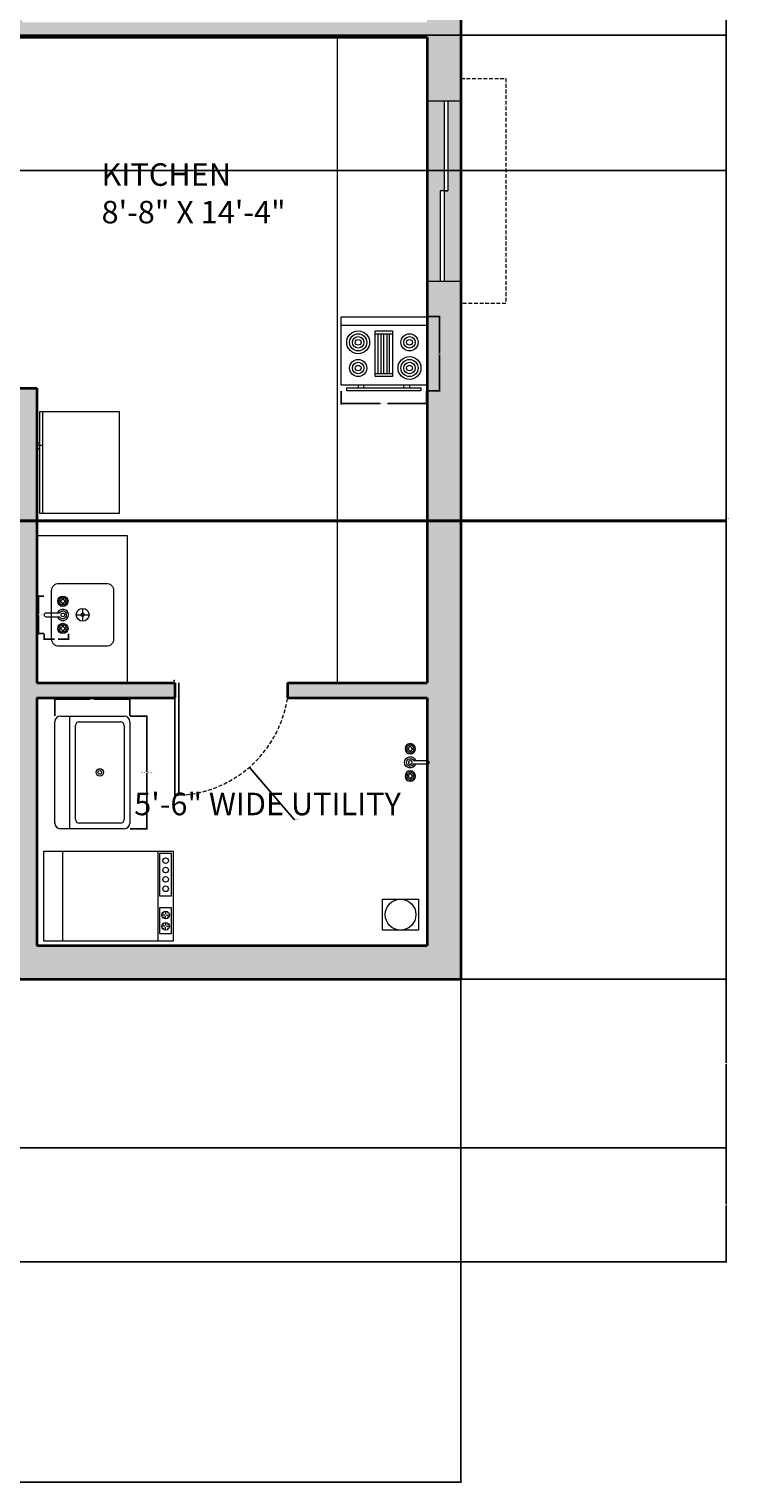
# Model space of a CAD drawing. Units: inches. Extents: x 1693 to 2974, y 2201 to 2965.
# Tile 19 of 24: x 2787 to 2974, y 2201 to 2588. Entities that reach past the tile are written whole.
import ezdxf

# ---------------------------------------------------------------- set-up
doc = ezdxf.new("R2010")
doc.units = ezdxf.units.IN
doc.header["$LTSCALE"] = 2
doc.header["$MEASUREMENT"] = 0
doc.linetypes.add('HIDDEN', pattern=[0.375, 0.25, -0.125])
for name, color, linetype, lineweight in [('A-ANNO-DIMS', 2, 'Continuous', 18), ('A-AREA-IDEN', 7, 'Continuous', 18), ('A-DOOR', 3, 'Continuous', 25), ('A-DOOR-SWNG', 3, 'HIDDEN', 13), ('A-EQPM', 8, 'Continuous', 18), ('A-FLOR-CASE', 32, 'Continuous', 18), ('A-FLOR-FIXT', 9, 'Continuous', 18), ('A-GLAZ', 4, 'Continuous', 18), ('A-GLAZ-OVHD', 8, 'HIDDEN', 13), ('A-WALL', 7, 'Continuous', 35)]:
    doc.layers.add(name, color=color, linetype=linetype, lineweight=lineweight)
doc.layers.add('A-GLAZ-PATT', color=141, linetype='Continuous', lineweight=13, true_color=0xadddf7)
doc.layers.add('A-WALL-PATT', color=251, linetype='Continuous', lineweight=13, true_color=0x636466)
doc.styles.get("Standard").update_dxf_attribs({"font": 'arial.ttf'})
doc.dimstyles.get("Standard").update_dxf_attribs({"dimtxt": 0.18, "dimasz": 0.18, "dimexe": 0.18, "dimexo": 0.0625, "dimgap": 0.09, "dimtad": 0, "dimtih": 1, "dimtoh": 1, "dimdec": 1, "dimzin": 0, "dimdsep": 46, "dimlunit": 3, "dimtxsty": 'Standard', "dimcen": 0.09, "dimadec": 0, "dimazin": 0, "dimtfac": 1, "dimtdec": 1, "dimtofl": 0, "dimtmove": 0, "dimatfit": 3, "dimfxl": 1, "dimtolj": 1, "dimtzin": 0, "dimarcsym": 0})

# ---------------------------------------------------------------- blocks, each defined once
blk = doc.blocks.new('Range-Oven - 30 in top')
for p, q in [((0, -3), (30, -3)), ((12, -6), (18, -6)), ((13, -20), (13, -6)), ((14, -6), (14, -20)), ((15, -20), (15, -6)), ((16, -6), (16, -20)), ((17, -20), (17, -6)), ((18, -20), (12, -20)), ((6, -24), (6, -25)), ((8, -25), (8, -24)), ((22, -25), (22, -24)), ((24, -24), (24, -25))]:
    blk.add_line(p, q)
for points in [[(0, -24), (0, 0), (30, 0), (30, -24)], [(12, -21), (12, -5), (18, -5), (18, -21)], [(2, -26), (2, -25), (28, -25), (28, -26)]]:
    blk.add_lwpolyline(points, close=True)
for centre, radius in [((6, -9), 4), ((6, -9), 3), ((6, -9), 2), ((6, -9), 1), ((24, -9), 3), ((24, -9), 2), ((24, -9), 1), ((6, -18), 3), ((24, -18), 4), ((24, -18), 3), ((6, -18), 2), ((6, -18), 1), ((24, -18), 2), ((24, -18), 1)]:
    blk.add_circle(centre, radius)
blk = doc.blocks.new('Dishwasher')
for p, q in [((16, 32.5), (16.75, 32.5)), ((16.5, 32), (16.2942, 31.7942)), ((16.3156, 33.1843), (16.5, 33)), ((17, 32.75), (17, 33.5)), ((17, 32.25), (17, 31.5)), ((18, 32.5), (17.25, 32.5)), ((17.5, 33), (17.6938, 33.1938)), ((17.7061, 31.7939), (17.5, 32)), ((19, 32.5), (19.75, 32.5)), ((19.5, 32), (19.2942, 31.7942)), ((19.3156, 33.1843), (19.5, 33)), ((20, 32.75), (20, 33.5)), ((20, 32.25), (20, 31.5)), ((21, 32.5), (20.25, 32.5)), ((20.5, 33), (20.6938, 33.1938)), ((20.7061, 31.7939), (20.5, 32)), ((24, 30.5), (0, 30.5)), ((0, 5), (24, 5))]:
    blk.add_line(p, q)
for points in [[(0, 0), (0, 34.5), (24, 34.5), (24, 0)], [(0.5, 31), (0.5, 34), (12, 34), (12, 31)], [(15, 31), (15, 34), (22, 34), (22, 31)]]:
    blk.add_lwpolyline(points, close=True)
for centre, radius in [((2.5, 32.5), 0.75), ((5, 32.5), 0.75), ((7.5, 32.5), 0.75), ((10, 32.5), 0.75), ((17, 32.5), 1), ((20, 32.5), 1)]:
    blk.add_circle(centre, radius)
blk = doc.blocks.new('Sink-single - 30 in top')
blk.add_line((-15, -3.999996), (15, -3.999996))
for points in [[(-13.5, 0), (13.5, 0)], [(-15, -18.499996), (-15, -1.5)], [(15, -1.5), (15, -18.499996)], [(-13.5, -17.499996), (-13.5, -6.499996)], [(-12.5, -5.499996), (12.5, -5.499996)], [(13.5, -6.499996), (13.5, -17.499996)], [(12.5, -18.499996), (-12.5, -18.499996)], [(13.5, -19.999996), (-13.5, -19.999996)]]:
    blk.add_lwpolyline(points)
for radius in [1, 0.5]:
    blk.add_circle((0, -11.999996), radius)
for centre, radius, start, end in [((-13.5, -1.5), 1.5, 90, 180), ((13.5, -1.5), 1.5, 0, 90), ((-12.5, -6.499996), 1, 90, 180), ((12.5, -6.499996), 1, 0, 90), ((-13.5, -18.499996), 1.5, 180, 270), ((-12.5, -17.499996), 1, 180, 270), ((12.5, -17.499996), 1, 270, 0), ((13.5, -18.499996), 1.5, 270, 0)]:
    blk.add_arc(centre, radius, start, end)
blk = doc.blocks.new('Faucet - Bathroom top')
for p, q in [((-4.107, 0.125), (-4.375, 0.125)), ((-3.75, 0.4788), (-3.75, 0.75)), ((-3.5, 0.482), (-3.5, 0.75)), ((-3.1461, 0.125), (-2.875, 0.125)), ((3.143, 0.125), (2.875, 0.125)), ((3.5, 0.4788), (3.5, 0.75)), ((3.75, 0.482), (3.75, 0.75)), ((4.1039, 0.125), (4.375, 0.125)), ((-4.1039, -0.125), (-4.375, -0.125)), ((-3.75, -0.4821), (-3.75, -0.75)), ((-3.5, -0.4789), (-3.5, -0.75)), ((-3.143, -0.125), (-2.875, -0.125)), ((-0.5, -0.8639), (-0.5, -4.5)), ((0.5, -4.5), (0.5, -0.8631)), ((3.1461, -0.125), (2.875, -0.125)), ((3.5, -0.4821), (3.5, -0.75)), ((3.75, -0.4789), (3.75, -0.75)), ((4.107, -0.125), (4.375, -0.125))]:
    blk.add_line(p, q)
for centre, radius in [((-3.625, 0), 1.375), ((-4.625, 0), 0.2795), ((-3.625, 0), 0.5), ((-3.625, 1), 0.2795), ((-2.625, 0), 0.2795), ((0, 0), 0.5), ((3.625, 0), 1.375), ((2.625, 0), 0.2795), ((3.625, 0), 0.5), ((3.625, 1), 0.2795), ((4.625, 0), 0.2795), ((-3.625, -1), 0.2795), ((3.625, -1), 0.2795)]:
    blk.add_circle(centre, radius)
for centre, radius, start, end in [((-3.625, 0), 1, 105.2407, 164.2093), ((-3.625, 0), 1, 16.44125, 74.07887), ((0, 0), 1.5, 289.6514, 250.3603), ((0, 0), 1, 300.3431, 239.7554), ((3.625, 0), 1, 106.12, 164.0884), ((3.625, 0), 1, 16.23422, 73.90469), ((-3.625, 0), 1, 196.2342, 253.9047), ((-3.625, 0), 1, 286.12, 344.0884), ((3.625, 0), 1, 196.4413, 254.0789), ((3.625, 0), 1, 285.2407, 344.2093), ((0, -4.5), 0.5, 180, 0)]:
    blk.add_arc(centre, radius, start, end)
blk = doc.blocks.new('Refrigerator-2 door - 36 in top')
for p, q in [((0, -26.999999), (36, -26.999999)), ((11, -27.999999), (11, -28.999999)), ((11, -28.999999), (13, -28.999999)), ((12, -26.999999), (12, -28.999999)), ((13, -28.999999), (13, -27.999999))]:
    blk.add_line(p, q)
blk.add_lwpolyline([(0, -27.999999), (0, 0), (36, 0), (36, -27.999999)], close=True)
blk = doc.blocks.new('DRAIN-UTILITY')
at = {"ltscale": 2}
blk.add_lwpolyline([(0, 8.21), (9.59, 8.21), (9.59, 0), (0, 0)], close=True, dxfattribs=at)
blk.add_circle((4.8, 4.1), 4.1, dxfattribs=at)
blk = doc.blocks.new('WINDOW-HOOD-60IN')
at = {"ltscale": 2}
for p, q in [((6, 12), (0, 12)), ((0, 12), (0, 0)), ((60, 12), (6, 12)), ((60, 0), (60, 12)), ((54, 0), (60, 0))]:
    blk.add_line(p, q, dxfattribs=at)
blk = doc.blocks.new('*D35')
at = {"layer": 'A-ANNO-DIMS', "color": 0, "lineweight": -2, "ltscale": 2, "transparency": 16777216}
for p, q in [((2791.07, 2436.84), (2789.46, 2436.84)), ((2789.64, 2436.66), (2789.64, 2432.02)), ((2789.64, 2427.02), (2789.64, 2431.66)), ((2791.07, 2426.84), (2789.46, 2426.84))]:
    blk.add_line(p, q, dxfattribs=at)
at = {"layer": 'A-ANNO-DIMS', "color": 0, "ltscale": 2, "transparency": 16777216}
for points in [[(2789.61, 2436.66), (2789.67, 2436.66), (2789.64, 2436.84)], [(2789.61, 2427.02), (2789.67, 2427.02), (2789.64, 2426.84)]]:
    blk.add_solid(points, dxfattribs=at)
at = {"layer": 'Defpoints', "color": 0, "ltscale": 2, "transparency": 16777216}
for p in [(2791.14, 2436.84), (2789.64, 2426.84), (2791.14, 2426.84)]:
    blk.add_point(p, dxfattribs=at)
at = {"layer": 'A-ANNO-DIMS', "color": 0, "ltscale": 2, "transparency": 16777216, "insert": (2789.64, 2431.84), "char_height": 0.18, "attachment_point": 5}
blk.add_mtext('\\A1;TAP - PLAN 10 TYP.', dxfattribs=at)
blk = doc.blocks.new('*D36')
at = {"layer": 'A-ANNO-DIMS', "color": 0, "lineweight": -2, "ltscale": 2, "transparency": 16777216}
for p, q in [((2791.14, 2426.78), (2791.14, 2425.16)), ((2791.32, 2425.34), (2793.93, 2425.34)), ((2797.46, 2425.34), (2794.84, 2425.34)), ((2797.64, 2426.78), (2797.64, 2425.16))]:
    blk.add_line(p, q, dxfattribs=at)
at = {"layer": 'A-ANNO-DIMS', "color": 0, "ltscale": 2, "transparency": 16777216}
for points in [[(2791.32, 2425.37), (2791.32, 2425.31), (2791.14, 2425.34)], [(2797.46, 2425.37), (2797.46, 2425.31), (2797.64, 2425.34)]]:
    blk.add_solid(points, dxfattribs=at)
at = {"layer": 'Defpoints', "color": 0, "ltscale": 2, "transparency": 16777216}
for p in [(2791.14, 2426.84), (2797.64, 2426.84), (2797.64, 2425.34)]:
    blk.add_point(p, dxfattribs=at)
at = {"layer": 'A-ANNO-DIMS', "color": 0, "ltscale": 2, "transparency": 16777216, "insert": (2794.39, 2425.34), "char_height": 0.18, "attachment_point": 5}
blk.add_mtext('\\A1;7 TYP.', dxfattribs=at)
blk = doc.blocks.new('*D53')
at = {"layer": 'A-ANNO-DIMS', "color": 0, "lineweight": -2, "ltscale": 2, "transparency": 16777216}
for p, q in [((2870.29, 2491.47), (2870.29, 2487.94)), ((2893.09, 2491.47), (2893.09, 2487.94)), ((2870.47, 2488.12), (2880.68, 2488.12)), ((2892.91, 2488.12), (2882.69, 2488.12))]:
    blk.add_line(p, q, dxfattribs=at)
at = {"layer": 'A-ANNO-DIMS', "color": 0, "ltscale": 2, "transparency": 16777216}
for points in [[(2870.47, 2488.15), (2870.47, 2488.09), (2870.29, 2488.12)], [(2892.91, 2488.15), (2892.91, 2488.09), (2893.09, 2488.12)]]:
    blk.add_solid(points, dxfattribs=at)
at = {"layer": 'Defpoints', "color": 0, "ltscale": 2, "transparency": 16777216}
for p in [(2870.29, 2491.54), (2893.09, 2491.54), (2893.09, 2488.12)]:
    blk.add_point(p, dxfattribs=at)
at = {"layer": 'A-ANNO-DIMS', "color": 0, "ltscale": 2, "transparency": 16777216, "insert": (2881.69, 2488.12), "char_height": 0.18, "attachment_point": 5}
blk.add_mtext('\\A1;RANGE 23 TYP.', dxfattribs=at)
blk = doc.blocks.new('*D54')
at = {"layer": 'A-ANNO-DIMS', "color": 0, "lineweight": -2, "ltscale": 2, "transparency": 16777216}
for p, q in [((2893.15, 2511.3), (2896.69, 2511.3)), ((2896.51, 2511.12), (2896.51, 2501.6)), ((2896.51, 2491.72), (2896.51, 2501.24)), ((2893.15, 2491.54), (2896.69, 2491.54))]:
    blk.add_line(p, q, dxfattribs=at)
at = {"layer": 'A-ANNO-DIMS', "color": 0, "ltscale": 2, "transparency": 16777216}
for points in [[(2896.48, 2511.12), (2896.54, 2511.12), (2896.51, 2511.3)], [(2896.48, 2491.72), (2896.54, 2491.72), (2896.51, 2491.54)]]:
    blk.add_solid(points, dxfattribs=at)
at = {"layer": 'Defpoints', "color": 0, "ltscale": 2, "transparency": 16777216}
for p in [(2893.09, 2511.3), (2896.51, 2511.3), (2893.09, 2491.54)]:
    blk.add_point(p, dxfattribs=at)
at = {"layer": 'A-ANNO-DIMS', "color": 0, "ltscale": 2, "transparency": 16777216, "insert": (2896.51, 2501.42), "char_height": 0.18, "attachment_point": 5}
blk.add_mtext('\\A1;20 TYP.', dxfattribs=at)
blk = doc.blocks.new('*D59')
at = {"layer": 'A-ANNO-DIMS', "color": 0, "lineweight": -2, "ltscale": 2, "transparency": 16777216}
for p, q in [((2814.04, 2404.86), (2818.66, 2404.86)), ((2818.48, 2404.68), (2818.48, 2390.05)), ((2818.48, 2375.04), (2818.48, 2389.68)), ((2814.04, 2374.86), (2818.66, 2374.86))]:
    blk.add_line(p, q, dxfattribs=at)
at = {"layer": 'A-ANNO-DIMS', "color": 0, "ltscale": 2, "transparency": 16777216}
for points in [[(2818.45, 2404.68), (2818.51, 2404.68), (2818.48, 2404.86)], [(2818.45, 2375.04), (2818.51, 2375.04), (2818.48, 2374.86)]]:
    blk.add_solid(points, dxfattribs=at)
at = {"layer": 'Defpoints', "color": 0, "ltscale": 2, "transparency": 16777216}
for p in [(2813.98, 2404.86), (2818.48, 2404.86), (2813.98, 2374.86)]:
    blk.add_point(p, dxfattribs=at)
at = {"layer": 'A-ANNO-DIMS', "color": 0, "ltscale": 2, "transparency": 16777216, "insert": (2818.48, 2389.86), "char_height": 0.18, "attachment_point": 5}
blk.add_mtext('\\A1;SINGLE-BOWL SINK 30 TYP.', dxfattribs=at)
blk = doc.blocks.new('*D60')
at = {"layer": 'A-ANNO-DIMS', "color": 0, "lineweight": -2, "ltscale": 2, "transparency": 16777216}
for p, q in [((2793.98, 2404.93), (2793.98, 2409.54)), ((2813.98, 2404.93), (2813.98, 2409.54)), ((2794.16, 2409.36), (2803.45, 2409.36)), ((2813.8, 2409.36), (2804.51, 2409.36))]:
    blk.add_line(p, q, dxfattribs=at)
at = {"layer": 'A-ANNO-DIMS', "color": 0, "ltscale": 2, "transparency": 16777216}
for points in [[(2794.16, 2409.39), (2794.16, 2409.33), (2793.98, 2409.36)], [(2813.8, 2409.39), (2813.8, 2409.33), (2813.98, 2409.36)]]:
    blk.add_solid(points, dxfattribs=at)
at = {"layer": 'Defpoints', "color": 0, "ltscale": 2, "transparency": 16777216}
for p in [(2793.98, 2409.36), (2793.98, 2404.86), (2813.98, 2404.86)]:
    blk.add_point(p, dxfattribs=at)
at = {"layer": 'A-ANNO-DIMS', "color": 0, "ltscale": 2, "transparency": 16777216, "insert": (2803.98, 2409.36), "char_height": 0.18, "attachment_point": 5}
blk.add_mtext('\\A1;20 TYP.', dxfattribs=at)
blk = doc.blocks.new('*D81')
at = {"layer": 'A-ANNO-DIMS', "color": 0, "lineweight": -2, "ltscale": 2, "transparency": 16777216}
for p, q in [((1752.34, 2553.91), (1752.34, 2964.96)), ((1752.52, 2964.78), (2332.94, 2964.78)), ((2914.06, 2964.78), (2333.64, 2964.78)), ((2914.24, 2754.97), (2914.24, 2964.96))]:
    blk.add_line(p, q, dxfattribs=at)
at = {"layer": 'A-ANNO-DIMS', "color": 0, "ltscale": 2, "transparency": 16777216}
for points in [[(1752.52, 2964.81), (1752.52, 2964.75), (1752.34, 2964.78)], [(2914.06, 2964.81), (2914.06, 2964.75), (2914.24, 2964.78)]]:
    blk.add_solid(points, dxfattribs=at)
at = {"layer": 'Defpoints', "color": 0, "ltscale": 2, "transparency": 16777216}
for p in [(2914.24, 2964.78), (2914.24, 2754.9), (1752.34, 2553.84)]:
    blk.add_point(p, dxfattribs=at)
at = {"layer": 'A-ANNO-DIMS', "color": 0, "ltscale": 2, "transparency": 16777216, "insert": (2333.29, 2964.78), "char_height": 0.18, "attachment_point": 5}
blk.add_mtext('\\A1;1162', dxfattribs=at)
blk = doc.blocks.new('*D85')
at = {"layer": 'A-ANNO-DIMS', "color": 0, "lineweight": -2, "ltscale": 2, "transparency": 16777216}
for p, q in [((2479.24, 2334.69), (2479.24, 2200.56)), ((2902.24, 2334.69), (2902.24, 2200.56)), ((2479.42, 2200.74), (2690.44, 2200.74)), ((2902.06, 2200.74), (2691.03, 2200.74))]:
    blk.add_line(p, q, dxfattribs=at)
at = {"layer": 'A-ANNO-DIMS', "color": 0, "ltscale": 2, "transparency": 16777216}
for points in [[(2479.42, 2200.77), (2479.42, 2200.71), (2479.24, 2200.74)], [(2902.06, 2200.77), (2902.06, 2200.71), (2902.24, 2200.74)]]:
    blk.add_solid(points, dxfattribs=at)
at = {"layer": 'Defpoints', "color": 0, "ltscale": 2, "transparency": 16777216}
for p in [(2479.24, 2334.75), (2902.24, 2334.75), (2902.24, 2200.74)]:
    blk.add_point(p, dxfattribs=at)
at = {"layer": 'A-ANNO-DIMS', "color": 0, "ltscale": 2, "transparency": 16777216, "insert": (2690.74, 2200.74), "char_height": 0.18, "attachment_point": 5}
blk.add_mtext('\\A1;423', dxfattribs=at)
blk = doc.blocks.new('*D87')
at = {"layer": 'A-ANNO-DIMS', "color": 0, "lineweight": -2, "ltscale": 2, "transparency": 16777216}
for p, q in [((2902.3, 2846.25), (2973.12, 2846.25)), ((2972.94, 2846.07), (2972.94, 2590.69)), ((2972.94, 2334.93), (2972.94, 2590.32)), ((2902.3, 2334.75), (2973.12, 2334.75))]:
    blk.add_line(p, q, dxfattribs=at)
at = {"layer": 'A-ANNO-DIMS', "color": 0, "ltscale": 2, "transparency": 16777216}
for points in [[(2972.91, 2846.07), (2972.97, 2846.07), (2972.94, 2846.25)], [(2972.91, 2334.93), (2972.97, 2334.93), (2972.94, 2334.75)]]:
    blk.add_solid(points, dxfattribs=at)
at = {"layer": 'Defpoints', "color": 0, "ltscale": 2, "transparency": 16777216}
for p in [(2902.24, 2846.25), (2972.94, 2846.25), (2902.24, 2334.75)]:
    blk.add_point(p, dxfattribs=at)
at = {"layer": 'A-ANNO-DIMS', "color": 0, "ltscale": 2, "transparency": 16777216, "insert": (2972.94, 2590.5), "char_height": 0.18, "attachment_point": 5}
blk.add_mtext('\\A1;511.5', dxfattribs=at)
blk = doc.blocks.new('*D89')
at = {"layer": 'A-ANNO-DIMS', "color": 0, "lineweight": -2, "ltscale": 2, "transparency": 16777216}
for p, q in [((2479.3, 2334.75), (2973.12, 2334.75)), ((2972.94, 2334.57), (2972.94, 2312.48)), ((2972.94, 2290.02), (2972.94, 2312.12)), ((2294.3, 2289.84), (2973.12, 2289.84))]:
    blk.add_line(p, q, dxfattribs=at)
at = {"layer": 'A-ANNO-DIMS', "color": 0, "ltscale": 2, "transparency": 16777216}
for points in [[(2972.91, 2334.57), (2972.97, 2334.57), (2972.94, 2334.75)], [(2972.91, 2290.02), (2972.97, 2290.02), (2972.94, 2289.84)]]:
    blk.add_solid(points, dxfattribs=at)
at = {"layer": 'Defpoints', "color": 0, "ltscale": 2, "transparency": 16777216}
for p in [(2479.24, 2334.75), (2972.94, 2334.75), (2294.24, 2289.84)]:
    blk.add_point(p, dxfattribs=at)
at = {"layer": 'A-ANNO-DIMS', "color": 0, "ltscale": 2, "transparency": 16777216, "insert": (2972.94, 2312.3), "char_height": 0.18, "attachment_point": 5}
blk.add_mtext('\\A1;44.91', dxfattribs=at)
blk = doc.blocks.new('*D95')
at = {"layer": 'A-ANNO-DIMS', "color": 0, "lineweight": -2, "ltscale": 2, "transparency": 16777216}
for p, q in [((2189.3, 2289.84), (2973.12, 2289.84)), ((2972.94, 2289.66), (2972.94, 2274.83)), ((2972.94, 2259.62), (2972.94, 2274.46)), ((2189.3, 2259.44), (2973.12, 2259.44))]:
    blk.add_line(p, q, dxfattribs=at)
at = {"layer": 'A-ANNO-DIMS', "color": 0, "ltscale": 2, "transparency": 16777216}
for points in [[(2972.91, 2289.66), (2972.97, 2289.66), (2972.94, 2289.84)], [(2972.91, 2259.62), (2972.97, 2259.62), (2972.94, 2259.44)]]:
    blk.add_solid(points, dxfattribs=at)
at = {"layer": 'Defpoints', "color": 0, "ltscale": 2, "transparency": 16777216}
for p in [(2189.24, 2289.84), (2972.94, 2289.84), (2189.24, 2259.44)]:
    blk.add_point(p, dxfattribs=at)
at = {"layer": 'A-ANNO-DIMS', "color": 0, "ltscale": 2, "transparency": 16777216, "insert": (2972.94, 2274.64), "char_height": 0.18, "attachment_point": 5}
blk.add_mtext('\\A1;30.4', dxfattribs=at)
blk = doc.blocks.new('*D96')
at = {"layer": 'A-ANNO-DIMS', "color": 0, "lineweight": -2, "ltscale": 2, "transparency": 16777216}
for p, q in [((2294.3, 2586.26), (2973.12, 2586.26)), ((2972.94, 2586.08), (2972.94, 2568.45)), ((2972.94, 2550.44), (2972.94, 2568.08)), ((2294.3, 2550.26), (2973.12, 2550.26))]:
    blk.add_line(p, q, dxfattribs=at)
at = {"layer": 'A-ANNO-DIMS', "color": 0, "ltscale": 2, "transparency": 16777216}
for points in [[(2972.91, 2586.08), (2972.97, 2586.08), (2972.94, 2586.26)], [(2972.91, 2550.44), (2972.97, 2550.44), (2972.94, 2550.26)]]:
    blk.add_solid(points, dxfattribs=at)
at = {"layer": 'Defpoints', "color": 0, "ltscale": 2, "transparency": 16777216}
for p in [(2294.24, 2586.26), (2972.94, 2586.26), (2294.24, 2550.26)]:
    blk.add_point(p, dxfattribs=at)
at = {"layer": 'A-ANNO-DIMS', "color": 0, "ltscale": 2, "transparency": 16777216, "insert": (2972.94, 2568.26), "char_height": 0.18, "attachment_point": 5}
blk.add_mtext('\\A1;36', dxfattribs=at)
blk = doc.blocks.new('*D97')
at = {"layer": 'A-ANNO-DIMS', "color": 0, "lineweight": -2, "ltscale": 2, "transparency": 16777216}
for p, q in [((2294.3, 2631.75), (2973.12, 2631.75)), ((2972.94, 2631.57), (2972.94, 2609.19)), ((2972.94, 2586.44), (2972.94, 2608.83)), ((2294.3, 2586.26), (2973.12, 2586.26))]:
    blk.add_line(p, q, dxfattribs=at)
at = {"layer": 'A-ANNO-DIMS', "color": 0, "ltscale": 2, "transparency": 16777216}
for points in [[(2972.91, 2631.57), (2972.97, 2631.57), (2972.94, 2631.75)], [(2972.91, 2586.44), (2972.97, 2586.44), (2972.94, 2586.26)]]:
    blk.add_solid(points, dxfattribs=at)
at = {"layer": 'Defpoints', "color": 0, "ltscale": 2, "transparency": 16777216}
for p in [(2294.24, 2631.75), (2972.94, 2631.75), (2294.24, 2586.26)]:
    blk.add_point(p, dxfattribs=at)
at = {"layer": 'A-ANNO-DIMS', "color": 0, "ltscale": 2, "transparency": 16777216, "insert": (2972.94, 2609.01), "char_height": 0.18, "attachment_point": 5}
blk.add_mtext('\\A1;45.49', dxfattribs=at)
blk = doc.blocks.new('*D108')
at = {"layer": 'A-ANNO-DIMS', "color": 0, "lineweight": -2, "ltscale": 2, "transparency": 16777216}
for p, q in [((1752.74, 2457.09), (2973.12, 2457.09)), ((1752.74, 2456.73), (2973.12, 2456.73)), ((2972.94, 2457.27), (2972.94, 2457.45)), ((2972.94, 2457.45), (2973.12, 2457.45)), ((2972.94, 2456.55), (2972.94, 2456.37))]:
    blk.add_line(p, q, dxfattribs=at)
at = {"layer": 'A-ANNO-DIMS', "color": 0, "ltscale": 2, "transparency": 16777216}
for points in [[(2972.91, 2457.27), (2972.97, 2457.27), (2972.94, 2457.09)], [(2972.91, 2456.55), (2972.97, 2456.55), (2972.94, 2456.73)]]:
    blk.add_solid(points, dxfattribs=at)
at = {"layer": 'Defpoints', "color": 0, "ltscale": 2, "transparency": 16777216}
for p in [(1752.68, 2457.09), (1752.68, 2456.73), (2972.94, 2457.09)]:
    blk.add_point(p, dxfattribs=at)
at = {"layer": 'A-ANNO-DIMS', "color": 0, "ltscale": 2, "transparency": 16777216, "insert": (2973.44, 2457.45), "char_height": 0.18, "attachment_point": 5}
blk.add_mtext('\\A1;0.36', dxfattribs=at)
blk = doc.blocks.new('*D119')
at = {"layer": 'A-ANNO-DIMS', "color": 0, "lineweight": -2, "ltscale": 2, "transparency": 16777216}
for p, q in [((2825.7, 2414.32), (2825.88, 2414.32)), ((2825.79, 2414.23), (2825.79, 2414.41)), ((2857.82, 2377.36), (2845.93, 2391.09)), ((2858, 2377.36), (2857.82, 2377.36))]:
    blk.add_line(p, q, dxfattribs=at)
at = {"layer": 'A-ANNO-DIMS', "color": 0, "ltscale": 2, "transparency": 16777216}
blk.add_solid([(2845.95, 2391.11), (2845.91, 2391.07), (2845.81, 2391.22)], dxfattribs=at)
at = {"layer": 'Defpoints', "color": 0, "ltscale": 2, "transparency": 16777216}
for p in [(2825.79, 2414.32), (2845.81, 2391.22)]:
    blk.add_point(p, dxfattribs=at)
at = {"layer": 'A-ANNO-DIMS', "color": 0, "ltscale": 2, "transparency": 16777216, "insert": (2858.55, 2377.36), "char_height": 0.18, "attachment_point": 5}
blk.add_mtext('\\A1;R30.567', dxfattribs=at)

msp = doc.modelspace()

# ---------------------------------------------------------------- hatches: boundary and pattern name
at = {"layer": 'A-GLAZ-PATT', "ltscale": 2}
h = msp.add_hatch(color=256, dxfattribs=at)
h.dxf.hatch_style = 1
h.paths.add_polyline_path([(2656.9702, 2338.2547), (2632.9702, 2338.2547), (2632.9702, 2339.2547), (2608.9702, 2339.2547), (2608.9702, 2334.7547), (2656.9702, 2334.7547)])
h.paths.add_polyline_path([(2656.9702, 2343.7547), (2608.9702, 2343.7547), (2608.9702, 2340.2547), (2632.9702, 2340.2547), (2632.9702, 2339.2547), (2656.9702, 2339.2547)])
h.paths.add_polyline_path([(2775.7544, 2338.2547), (2751.7544, 2338.2547), (2751.7544, 2334.7547), (2775.7544, 2334.7547)])
h.paths.add_polyline_path([(2775.7544, 2343.7547), (2751.7544, 2343.7547), (2751.7544, 2340.2547), (2775.7544, 2340.2547)])
h.paths.add_polyline_path([(2897.7363, 2568.7999), (2893.2363, 2568.7999), (2893.2363, 2520.7999), (2896.7363, 2520.7999), (2896.7363, 2544.7999), (2897.7363, 2544.7999)])
h.paths.add_polyline_path([(2902.2363, 2568.7999), (2898.7363, 2568.7999), (2898.7363, 2544.7999), (2897.7363, 2544.7999), (2897.7363, 2520.7999), (2902.2363, 2520.7999)])
h.paths.add_polyline_path([(2902.2363, 2637.7547), (2898.7363, 2637.7547), (2898.7363, 2613.7547), (2902.2363, 2613.7547)])
h.paths.add_polyline_path([(2896.7363, 2637.7547), (2893.2363, 2637.7547), (2893.2363, 2613.7547), (2896.7363, 2613.7547)])
h.paths.add_polyline_path([(2902.2363, 2748.903), (2899.0477, 2748.903), (2899.0477, 2724.903), (2898.0477, 2724.903), (2898.0477, 2700.903), (2902.2363, 2700.903)])
h.paths.add_polyline_path([(2898.0477, 2748.903), (2893.2363, 2748.903), (2893.2363, 2700.903), (2897.0477, 2700.903), (2897.0477, 2724.903), (2898.0477, 2724.903)])
h.paths.add_polyline_path([(2851.2363, 2846.2547), (2803.2363, 2846.2547), (2803.2363, 2842.7547), (2827.2363, 2842.7547), (2827.2363, 2841.7547), (2851.2363, 2841.7547)])
h.paths.add_polyline_path([(2851.2363, 2840.7547), (2827.2363, 2840.7547), (2827.2363, 2841.7547), (2803.2363, 2841.7547), (2803.2363, 2837.2547), (2851.2363, 2837.2547)])
h.paths.add_polyline_path([(2578.2363, 2846.2547), (2530.2363, 2846.2547), (2530.2363, 2842.7547), (2554.2363, 2842.7547), (2554.2363, 2841.7547), (2578.2363, 2841.7547)])
h.paths.add_polyline_path([(2578.2363, 2840.7547), (2554.2363, 2840.7547), (2554.2363, 2841.7547), (2530.2363, 2841.7547), (2530.2363, 2837.2547), (2578.2363, 2837.2547)])
h.paths.add_polyline_path([(2732.7363, 2812.7547), (2705.1363, 2812.7547), (2705.1363, 2811.7547), (2676.3363, 2811.7547), (2676.3363, 2812.7547), (2648.7363, 2812.7547), (2648.7363, 2808.2547), (2732.7363, 2808.2547)])
h.paths.add_polyline_path([(2732.7363, 2817.2547), (2648.7363, 2817.2547), (2648.7363, 2813.7547), (2676.3363, 2813.7547), (2676.3363, 2812.7547), (2705.1363, 2812.7547), (2705.1363, 2813.7547), (2732.7363, 2813.7547)])
h.paths.add_polyline_path([(2488.2363, 2695.8203), (2484.7878, 2695.8203), (2484.7878, 2671.8203), (2488.2363, 2671.8203)])
h.paths.add_polyline_path([(2482.7878, 2695.8203), (2479.2363, 2695.8203), (2479.2363, 2671.8203), (2482.7878, 2671.8203)])
h.paths.add_polyline_path([(2488.2363, 2572.4371), (2484.7363, 2572.4371), (2484.7363, 2541.4371), (2483.7363, 2541.4371), (2483.7363, 2512.4371), (2488.2363, 2512.4371)])
h.paths.add_polyline_path([(2482.7363, 2541.4371), (2483.7363, 2541.4371), (2483.7363, 2572.4371), (2479.2363, 2572.4371), (2479.2363, 2512.4371), (2482.7363, 2512.4371)])
h.paths.add_polyline_path([(2248.9863, 2706.8449), (2190.9863, 2706.8449), (2190.9863, 2703.3449), (2219.9863, 2703.3449), (2219.9863, 2702.3449), (2248.9863, 2702.3449)])
h.paths.add_polyline_path([(2248.9863, 2701.3449), (2219.9863, 2701.3449), (2219.9863, 2702.3449), (2190.9863, 2702.3449), (2190.9863, 2697.8449), (2248.9863, 2697.8449)])
h.paths.add_polyline_path([(2151.9207, 2293.3449), (2127.9207, 2293.3449), (2127.9207, 2289.8449), (2151.9207, 2289.8449)])
h.paths.add_polyline_path([(2151.9207, 2298.8449), (2127.9207, 2298.8449), (2127.9207, 2295.3449), (2151.9207, 2295.3449)])
h.paths.add_polyline_path([(2084.023, 2293.3449), (2066.023, 2293.3449), (2066.023, 2294.3449), (2048.023, 2294.3449), (2048.023, 2289.8449), (2084.023, 2289.8449)])
h.paths.add_polyline_path([(2084.023, 2298.8449), (2048.023, 2298.8449), (2048.023, 2295.3449), (2066.023, 2295.3449), (2066.023, 2294.3449), (2084.023, 2294.3449)])
h.paths.add_polyline_path([(1966.0781, 2293.3449), (1948.0781, 2293.3449), (1948.0781, 2294.3449), (1930.0781, 2294.3449), (1930.0781, 2289.8449), (1966.0781, 2289.8449)])
h.paths.add_polyline_path([(1966.0781, 2298.8449), (1930.0781, 2298.8449), (1930.0781, 2295.3449), (1948.0781, 2295.3449), (1948.0781, 2294.3449), (1966.0781, 2294.3449)])
h.paths.add_polyline_path([(1787.2363, 2403.1922), (1782.7363, 2403.1922), (1782.7363, 2355.1922), (1786.2363, 2355.1922), (1786.2363, 2379.1922), (1787.2363, 2379.1922)])
h.paths.add_polyline_path([(1791.7363, 2403.1922), (1788.2363, 2403.1922), (1788.2363, 2379.1922), (1787.2363, 2379.1922), (1787.2363, 2355.1922), (1791.7363, 2355.1922)])
h.paths.add_polyline_path([(1786.2363, 2477.5455), (1782.7363, 2477.5455), (1782.7363, 2453.5455), (1786.2363, 2453.5455)])
h.paths.add_polyline_path([(1791.7363, 2477.5455), (1788.2363, 2477.5455), (1788.2363, 2453.5455), (1791.7363, 2453.5455)])
h.paths.add_polyline_path([(1786.2363, 2621.6433), (1782.7363, 2621.6433), (1782.7363, 2585.6433), (1786.2363, 2585.6433)])
h.paths.add_polyline_path([(1791.7363, 2621.6433), (1788.2363, 2621.6433), (1788.2363, 2585.6433), (1791.7363, 2585.6433)])
h.paths.add_polyline_path([(1908.1286, 2706.8449), (1860.1286, 2706.8449), (1860.1286, 2703.3449), (1884.1286, 2703.3449), (1884.1286, 2702.3449), (1908.1286, 2702.3449)])
h.paths.add_polyline_path([(1908.1286, 2701.3449), (1884.1286, 2701.3449), (1884.1286, 2702.3449), (1860.1286, 2702.3449), (1860.1286, 2697.8449), (1908.1286, 2697.8449)])
h.paths.add_polyline_path([(1973.9863, 2706.8449), (1949.9863, 2706.8449), (1949.9863, 2703.3449), (1973.9863, 2703.3449)])
h.paths.add_polyline_path([(1973.9863, 2701.3449), (1949.9863, 2701.3449), (1949.9863, 2697.8449), (1973.9863, 2697.8449)])
h.paths.add_polyline_path([(2112.7363, 2690.3449), (2028.7363, 2690.3449), (2028.7363, 2686.8449), (2056.3363, 2686.8449), (2056.3363, 2685.8449), (2085.1363, 2685.8449), (2085.1363, 2686.8449), (2112.7363, 2686.8449)])
h.paths.add_polyline_path([(2112.7363, 2685.8449), (2085.1363, 2685.8449), (2085.1363, 2684.8449), (2056.3363, 2684.8449), (2056.3363, 2685.8449), (2028.7363, 2685.8449), (2028.7363, 2681.3449), (2112.7363, 2681.3449)])
h.paths.add_polyline_path([(2422.7363, 2640.7547), (2350.7363, 2640.7547), (2350.7363, 2637.2547), (2386.7363, 2637.2547), (2386.7363, 2636.2547), (2422.7363, 2636.2547)])
h.paths.add_polyline_path([(2422.7363, 2635.2547), (2386.7363, 2635.2547), (2386.7363, 2636.2547), (2350.7363, 2636.2547), (2350.7363, 2631.7547), (2422.7363, 2631.7547)])
at = {"layer": 'A-WALL-PATT', "ltscale": 2}
h = msp.add_hatch(color=256, dxfattribs=at)
h.dxf.hatch_style = 1
h.paths.add_polyline_path([(1928.2363, 2733.2161), (1930.9384, 2733.2161), (1930.9384, 2737.2161), (1923.7363, 2737.2161), (1923.7363, 2706.8449), (1908.1286, 2706.8449), (1908.1286, 2697.8449), (1923.7363, 2697.8449), (1923.7363, 2692.8449), (1928.2363, 2692.8449), (1928.2363, 2697.8449), (1949.9863, 2697.8449), (1949.9863, 2706.8449), (1928.2363, 2706.8449)])
h.paths.add_polyline_path([(2004.7363, 2737.2161), (1995.7363, 2737.2161), (1995.7363, 2706.8449), (1985.6374, 2706.8449), (1973.9863, 2706.8449), (1973.9863, 2697.8449), (2000.2363, 2697.8449), (2000.2363, 2686.5348), (2000.3613, 2686.5348), (2000.3613, 2667.0432), (2000.2363, 2601.8449), (1928.2363, 2601.8449), (1928.2363, 2662.8449), (1923.7363, 2662.8449), (1923.7363, 2595.3449), (1928.2363, 2595.3449), (1928.2363, 2597.3449), (2004.7363, 2597.3449), (2004.7363, 2681.3449), (2012.7814, 2681.3449), (2028.7363, 2681.3449), (2028.7363, 2690.3449), (2004.7363, 2690.3449)])
h.paths.add_polyline_path([(2190.9863, 2706.8449), (2184.9863, 2706.8449), (2145.7363, 2706.8449), (2145.7363, 2765.3449), (2145.7363, 2774.5394), (2136.7363, 2774.5394), (2136.7363, 2756.3449), (2136.7363, 2690.3449), (2112.7363, 2690.3449), (2112.7363, 2681.3449), (2136.7363, 2681.3449), (2136.7363, 2597.3449), (2141.2363, 2597.3449), (2141.2363, 2697.8449), (2190.9863, 2697.8449)])
h.paths.add_polyline_path([(1860.1286, 2706.8449), (1782.7363, 2706.8449), (1782.7363, 2621.6433), (1791.7363, 2621.6433), (1791.7363, 2697.8449), (1860.1286, 2697.8449)])
h.paths.add_polyline_path([(1791.7363, 2585.6433), (1782.7363, 2585.6433), (1782.7363, 2562.8449), (1782.7363, 2553.8449), (1752.3363, 2553.8449), (1752.3363, 2544.2586), (1756.3363, 2544.2586), (1756.3363, 2549.3449), (1782.7363, 2549.3449), (1782.7363, 2489.2404), (1782.7363, 2477.5455), (1791.7363, 2477.5455), (1791.7363, 2493.5991), (1791.6113, 2493.5991), (1791.6113, 2513.0907), (1791.6824, 2533.7198, -0.94742783), (1791.7363, 2534.7168), (1791.7363, 2549.3449), (1863.7363, 2549.3449), (1863.7363, 2513.3449), (1866.7363, 2513.3449), (1866.7363, 2549.3449), (1924.7363, 2549.3449), (1924.7363, 2447.3449), (1924.7363, 2442.8449), (1933.7363, 2442.8449), (1933.7363, 2447.3449), (1928.2363, 2447.3449), (1928.2363, 2559.3449), (1923.7363, 2559.3449), (1923.7363, 2553.8449), (1791.7363, 2553.8449), (1791.7363, 2562.8449)])
h.paths.add_polyline_path([(1791.7363, 2442.8449), (1866.7363, 2442.8449), (1866.7363, 2447.3449), (1866.7363, 2483.3449), (1863.7363, 2483.3449), (1863.7363, 2447.3449), (1791.7363, 2447.3449), (1791.7363, 2453.5455), (1782.7363, 2453.5455), (1782.7363, 2447.3449), (1756.3363, 2447.3449), (1756.3363, 2455.7126), (1752.3363, 2455.7126), (1752.3363, 2442.8449), (1782.7363, 2442.8449), (1782.7363, 2403.1922), (1791.7363, 2403.1922)])
h.paths.add_polyline_path([(1930.0781, 2298.8449), (1791.7363, 2298.8449), (1791.7363, 2355.1922), (1782.7363, 2355.1922), (1782.7363, 2289.8449), (1930.0781, 2289.8449)])
h.paths.add_polyline_path([(2624.7363, 2883.2547), (2624.7363, 2902.6165), (2624.7363, 2906.0761), (2615.7363, 2906.0761), (2615.7363, 2892.2547), (2615.7363, 2846.2547), (2578.2363, 2846.2547), (2578.2363, 2837.2547), (2620.2363, 2837.2547), (2620.2363, 2743.2547), (2624.7363, 2743.2547), (2624.7363, 2808.2547), (2648.7363, 2808.2547), (2648.7363, 2817.2547), (2624.7363, 2817.2547)])
h.paths.add_polyline_path([(2530.2363, 2846.2547), (2479.2363, 2846.2547), (2479.2363, 2695.8203), (2488.2363, 2695.8203), (2488.2363, 2700.7547), (2567.2363, 2700.7547), (2567.2363, 2705.2547), (2488.2363, 2705.2547), (2488.2363, 2837.2547), (2530.2363, 2837.2547)])
h.paths.add_polyline_path([(2488.2363, 2487.7547), (2630.2363, 2487.7547, -0.00990191), (2630.2363, 2489.0322), (2630.2363, 2492.2547), (2488.2363, 2492.2547), (2488.2363, 2512.4371), (2479.2363, 2512.4371), (2479.2363, 2334.7547), (2608.9702, 2334.7547), (2608.9702, 2343.7547), (2488.2363, 2343.7547)])
h.paths.add_polyline_path([(2751.7544, 2343.7547), (2672.7363, 2343.7547), (2672.7363, 2409.7547), (2674.7363, 2409.7547), (2674.7363, 2413.7547), (2672.7363, 2413.7547), (2672.7363, 2487.7547), (2732.7363, 2487.7547), (2732.7363, 2413.7547), (2704.7363, 2413.7547), (2704.7363, 2409.7547), (2784.7363, 2409.7547), (2784.7363, 2343.7547), (2775.7544, 2343.7547), (2775.7544, 2334.7547), (2902.2363, 2334.7547), (2902.2363, 2520.7999), (2893.2363, 2520.7999), (2893.2363, 2413.7547), (2856.0145, 2413.7547), (2856.0145, 2409.7547), (2893.2363, 2409.7547), (2893.2363, 2343.7547), (2789.2363, 2343.7547), (2789.2363, 2409.7547), (2819.2363, 2409.7547), (2826.0145, 2409.7547), (2826.0145, 2413.7547), (2789.2363, 2413.7547), (2789.2363, 2492.2547), (2784.7363, 2492.2547), (2784.7363, 2413.7547), (2736.7363, 2413.7547), (2736.7363, 2492.2547), (2672.7363, 2492.2547), (2666.2363, 2492.2547), (2666.2363, 2487.7547), (2668.2363, 2487.7547), (2668.2363, 2343.7547), (2656.9702, 2343.7547), (2656.9702, 2334.7547), (2662.9702, 2334.7547), (2751.7544, 2334.7547)])
h.paths.add_polyline_path([(2902.2363, 2613.7547), (2893.2363, 2613.7547), (2893.2363, 2589.7547), (2785.2363, 2589.7547), (2785.2363, 2661.7547), (2790.2363, 2661.7547), (2790.2363, 2665.2547), (2761.2363, 2665.2547), (2761.2363, 2667.2547), (2756.7363, 2667.2547), (2756.7363, 2661.7547), (2781.2363, 2661.7547), (2781.2363, 2585.7547), (2893.2363, 2585.7547), (2893.2363, 2568.7999), (2902.2363, 2568.7999)])
h.paths.add_polyline_path([(2488.2363, 2671.8203), (2479.2363, 2671.8203), (2479.2363, 2645.2547), (2479.2363, 2623.4598), (2488.2363, 2623.4598), (2488.2363, 2636.2547), (2624.7363, 2636.2547), (2624.7363, 2640.7547), (2603.7363, 2640.7547), (2603.7363, 2700.7547), (2624.7363, 2700.7547), (2624.7363, 2707.2547), (2620.2363, 2707.2547), (2620.2363, 2705.2547), (2597.2363, 2705.2547), (2597.2363, 2700.7547), (2599.2363, 2700.7547), (2599.2363, 2640.7547), (2488.2363, 2640.7547)])
h.paths.add_polyline_path([(2761.2363, 2837.2547), (2803.2363, 2837.2547), (2803.2363, 2846.2547), (2797.2363, 2846.2547), (2765.7363, 2846.2547), (2756.7363, 2846.2547), (2756.7363, 2817.2547), (2732.7363, 2817.2547), (2732.7363, 2808.2547), (2756.7363, 2808.2547), (2756.7363, 2703.2547), (2761.2363, 2703.2547)])
h.paths.add_polyline_path([(2739.7489, 2433.1234), (2786.9181, 2433.1234), (2786.9181, 2455.5122), (2739.7489, 2455.5122)], flags=25)

# ---------------------------------------------------------------- linework, layer by layer
at = {"layer": 'A-DOOR', "ltscale": 2}
for p, q in [((2826.0145, 2413.7547), (2826.0145, 2383.7547)), ((2827.0145, 2413.7547), (2827.0145, 2383.7547))]:
    msp.add_line(p, q, dxfattribs=at)
at = {"layer": 'A-DOOR-SWNG', "ltscale": 2}
msp.add_arc((2825.7908, 2414.3205), 30.5667, 270.419369, 351.409397, dxfattribs=at)
at = {"layer": 'A-FLOR-CASE'}
for p, q in [((2869.2363, 2585.7547), (2869.2363, 2413.7547)), ((2813.2363, 2453.0047), (2813.2363, 2413.7547))]:
    msp.add_line(p, q, dxfattribs=at)
at = {"layer": 'A-FLOR-CASE', "ltscale": 2}
msp.add_line((2789.2363, 2453.0047), (2813.2363, 2453.0047), dxfattribs=at)
at = {"layer": 'A-FLOR-FIXT', "ltscale": 2}
for p, q in [((2801.4038, 2433.5552), (2801.4038, 2430.1624)), ((2799.7074, 2431.8588), (2803.1002, 2431.8588))]:
    msp.add_line(p, q, dxfattribs=at)
msp.add_lwpolyline([(2795.1387, 2440.2493), (2807.6689, 2440.2493, -0.41421356), (2809.6689, 2438.2493), (2809.6689, 2425.4683, -0.41421356), (2807.6689, 2423.4683), (2795.1387, 2423.4683, -0.41421356), (2793.1387, 2425.4683), (2793.1387, 2438.2493, -0.41421356)], format="xyb", close=True, dxfattribs=at)
for radius in [1.6964, 0.4868]:
    msp.add_circle((2801.4038, 2431.8588), radius, dxfattribs=at)
at = {"layer": 'A-GLAZ', "ltscale": 2}
for p, q in [((2893.2363, 2568.7999), (2902.2363, 2568.7999)), ((2897.7363, 2568.7999), (2897.7363, 2520.7999)), ((2898.7363, 2568.7999), (2898.7363, 2544.7999)), ((2896.7363, 2544.7999), (2896.7363, 2520.7999)), ((2898.7363, 2544.7999), (2896.7363, 2544.7999)), ((2897.7363, 2544.7999), (2898.7363, 2544.7999)), ((2893.2363, 2520.7999), (2902.2363, 2520.7999))]:
    msp.add_line(p, q, dxfattribs=at)
at = {"layer": 'A-WALL'}
for p, q in [((2902.2363, 2846.2547), (2902.2363, 2334.7547)), ((2893.2363, 2585.7547), (2893.2363, 2413.7547)), ((2789.2363, 2492.2547), (2789.2363, 2413.7547)), ((2789.2363, 2409.7547), (2789.2363, 2343.7547)), ((2789.2363, 2409.7547), (2819.2363, 2409.7547)), ((2893.2363, 2409.7547), (2893.2363, 2343.7547))]:
    msp.add_line(p, q, dxfattribs=at)
at = {"layer": 'A-WALL', "ltscale": 2}
for p, q in [((2781.2363, 2585.7547), (2893.2363, 2585.7547)), ((2784.7363, 2492.2547), (2789.2363, 2492.2547)), ((2789.2363, 2413.7547), (2826.0145, 2413.7547)), ((2826.0145, 2413.7547), (2826.0145, 2409.7547)), ((2856.0145, 2413.7547), (2856.0145, 2409.7547)), ((2856.0145, 2413.7547), (2893.2363, 2413.7547)), ((2789.2363, 2409.7547), (2826.0145, 2409.7547)), ((2856.0145, 2409.7547), (2893.2363, 2409.7547)), ((2789.2363, 2343.7547), (2893.2363, 2343.7547)), ((2479.2363, 2334.7547), (2902.2363, 2334.7547))]:
    msp.add_line(p, q, dxfattribs=at)

# ---------------------------------------------------------------- block references
at = {"layer": 'A-EQPM', "ltscale": 2, "xscale": 0.7601168214309315, "yscale": 0.7601168214309315, "zscale": 0.7601168214309315}
msp.add_blockref('Range-Oven - 30 in top', (2870.2858, 2511.2993), dxfattribs=at)
at = {"layer": 'A-EQPM', "ltscale": 2, "xscale": 0.7541930673648309, "yscale": 0.7541930673648309, "zscale": 0.7541930673648309, "rotation": 270}
msp.add_blockref('Refrigerator-2 door - 36 in top', (2811.1079, 2485.9998), dxfattribs=at)
at = {"layer": 'A-EQPM', "ltscale": 2, "rotation": 270}
msp.add_blockref('Dishwasher', (2791.0215, 2368.8671), dxfattribs=at)
at = {"layer": 'A-FLOR-FIXT', "ltscale": 2}
for name, p, rotation in [('Faucet - Bathroom top', (2796.1367, 2431.8424), 270), ('Sink-single - 30 in top', (2793.977, 2389.8626), 90)]:
    msp.add_blockref(name, p, dxfattribs=dict(at, rotation=rotation))
at = {"layer": 'A-FLOR-FIXT', "ltscale": 2, "xscale": -1, "rotation": 90}
msp.add_blockref('Faucet - Bathroom top', (2888.7363, 2392.534), dxfattribs=at)
at = {"layer": 'A-FLOR-FIXT'}
msp.add_blockref('DRAIN-UTILITY', (2881.333, 2347.8744), dxfattribs=at)
at = {"layer": 'A-GLAZ-OVHD', "extrusion": (0, 0, -1), "zscale": -1, "rotation": 89.99999999999973}
msp.add_blockref('WINDOW-HOOD-60IN', (-2902.2364, 2514.8002), dxfattribs=at)

# ---------------------------------------------------------------- texts
at = {"layer": 'A-AREA-IDEN', "ltscale": 2, "char_height": 6, "attachment_point": 1}
for s, insert in [('KITCHEN\\P8\'-8" X 14\'-4"', (2806.4454, 2552.1606)), ('5\'-6" WIDE UTILITY', (2815.1428, 2384.463))]:
    msp.add_mtext_dynamic_manual_height_columns(s, width=108.452746, gutter_width=1, heights=[0], dxfattribs=dict(at, insert=insert))

# ---------------------------------------------------------------- dimensions: what is measured, and where the dimension line sits
at = {"layer": 'A-ANNO-DIMS', "ltscale": 2}
for base, p1, p2, picture, middle in [((2914.2363, 2964.7761), (1752.3363, 2553.8449), (2914.2363, 2754.903), '*D81', (2333.2863, 2964.7761)), ((2902.2363, 2200.7449), (2479.2363, 2334.7547), (2902.2363, 2334.7547), '*D85', (2690.7363, 2200.7449))]:
    dim = msp.add_linear_dim(base=base, p1=p1, p2=p2, dimstyle='Standard', override={"dimdec": 0, "dimlfac": 1, "dimrnd": 0, "dimzin": 0, "dimdsep": 46, "dimlunit": 2}, dxfattribs=at)
    dim.commit()
    dim.dimension.update_dxf_attribs({"geometry": picture, "text_midpoint": middle})
for base, p1, p2, override, picture, middle in [((2972.9363, 2846.2547), (2902.2363, 2334.7547), (2902.2363, 2846.2547), {"dimdec": 1, "dimlfac": 1, "dimrnd": 0, "dimzin": 0, "dimdsep": 46, "dimlunit": 2}, '*D87', (2972.9363, 2590.5047)), ((2972.9363, 2631.7547), (2294.2363, 2586.2648), (2294.2363, 2631.7547), {"dimdec": 2, "dimlfac": 1, "dimrnd": 0, "dimzin": 0, "dimdsep": 46, "dimlunit": 2}, '*D97', (2972.9363, 2609.0097)), ((2972.9363, 2586.2648), (2294.2363, 2550.2648), (2294.2363, 2586.2648), {"dimdec": 0, "dimlfac": 1, "dimrnd": 0, "dimzin": 0, "dimdsep": 46, "dimlunit": 2}, '*D96', (2972.9363, 2568.2648)), ((2972.9363, 2457.0877), (1752.6754, 2456.7302), (1752.6754, 2457.0877), {"dimdec": 2, "dimlfac": 1, "dimrnd": 0, "dimzin": 0, "dimdsep": 46, "dimlunit": 2}, '*D108', (2973.44, 2457.4477)), ((2972.9363, 2334.7547), (2294.2363, 2289.8449), (2479.2363, 2334.7547), {"dimdec": 2, "dimlfac": 1, "dimrnd": 0, "dimzin": 0, "dimdsep": 46, "dimlunit": 2}, '*D89', (2972.9363, 2312.2998)), ((2972.9363, 2289.8449), (2189.2363, 2259.4449), (2189.2363, 2289.8449), {"dimdec": 1, "dimlfac": 1, "dimrnd": 0, "dimzin": 0, "dimdsep": 46, "dimlunit": 2}, '*D95', (2972.9363, 2274.6449))]:
    dim = msp.add_linear_dim(base=base, p1=p1, p2=p2, angle=90, dimstyle='Standard', override=override, dxfattribs=at)
    dim.commit()
    dim.dimension.update_dxf_attribs({"geometry": picture, "text_midpoint": middle})
for base, p1, p2, angle, text, picture, middle in [((2896.5098, 2511.2993), (2893.0893, 2491.5362), (2893.0893, 2511.2993), 90, '<> TYP.', '*D54', (2896.5098, 2501.4177)), ((2789.6367, 2426.8424), (2791.1367, 2436.8424), (2791.1367, 2426.8424), 270, 'TAP - PLAN <> TYP.', '*D35', (2789.6367, 2431.8424)), ((2793.977, 2409.3626), (2813.977, 2404.8626), (2793.977, 2404.8626), 180, '<> TYP.', '*D60', (2803.977, 2409.3626)), ((2818.477, 2404.8626), (2813.977, 2374.8626), (2813.977, 2404.8626), 90, 'SINGLE-BOWL SINK <> TYP.', '*D59', (2818.477, 2389.8626))]:
    dim = msp.add_linear_dim(base=base, p1=p1, p2=p2, angle=angle, text=text, dimstyle='Standard', override={"dimdec": 0, "dimlfac": 1, "dimrnd": 0, "dimzin": 0, "dimdsep": 46, "dimlunit": 2}, dxfattribs=at)
    dim.commit()
    dim.dimension.update_dxf_attribs({"geometry": picture, "text_midpoint": middle})
for base, p1, p2, text, picture, middle in [((2893.0893, 2488.1157), (2870.2858, 2491.5362), (2893.0893, 2491.5362), 'RANGE <> TYP.', '*D53', (2881.6876, 2488.1157)), ((2797.6368, 2425.3424), (2791.1367, 2426.8424), (2797.6368, 2426.8424), '<> TYP.', '*D36', (2794.3867, 2425.3424))]:
    dim = msp.add_linear_dim(base=base, p1=p1, p2=p2, text=text, dimstyle='Standard', override={"dimdec": 0, "dimlfac": 1, "dimrnd": 0, "dimzin": 0, "dimdsep": 46, "dimlunit": 2}, dxfattribs=at)
    dim.commit()
    dim.dimension.update_dxf_attribs({"geometry": picture, "text_midpoint": middle})
dim = msp.add_radius_dim(center=(2825.7908, 2414.3205), mpoint=(2845.8101, 2391.2219), dimstyle='Standard', override={"dimdec": 3, "dimlfac": 1, "dimrnd": 0, "dimzin": 0, "dimdsep": 46, "dimlunit": 2}, dxfattribs=at)
dim.commit()
dim.dimension.update_dxf_attribs({"geometry": '*D119', "text_midpoint": (2858.5514, 2377.3627), "dimtype": 164})

doc.saveas('drawing.dxf')
